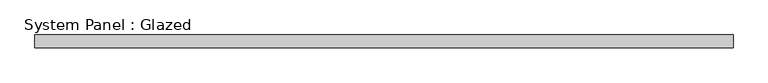
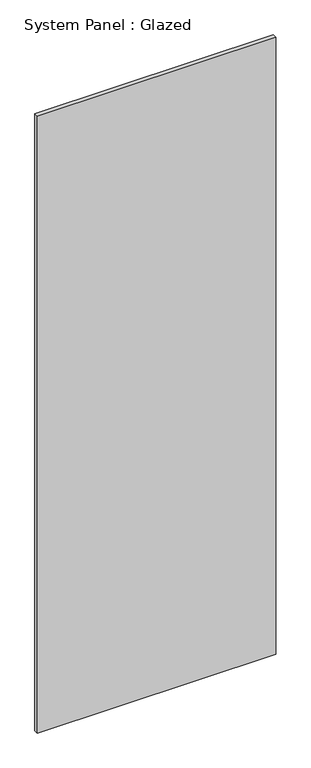
"""IFC4 building model written with IfcOpenShell, lengths in millimetres: plate geometry, System Panel : Glazed."""

from ifc_helpers import new_model, si_unit, origin, origin_with_axes, place, context, project, spatial, polyline, outline, extrude, source, transform, mapped, element, save


def system_panel_glazed_b761a9a7(model_context):
    return source(origin(), model_context, "Body", "SweptSolid", [
        extrude(outline(polyline([(698.5, 19.05), (-698.5, 19.05), (-698.5, 44.45), (698.5, 44.45), (698.5, 19.05)])), origin_with_axes(), (0.0, 0.0, 1.0), 3824.2205189),
    ])


if __name__ == "__main__":
    model = new_model("IFC4")
    model_context = context("Model", 3, world=origin())
    ifc_project = project(units=[si_unit("LENGTHUNIT", "METRE", prefix="MILLI")], contexts=[model_context])
    site = spatial("IfcSite", under=ifc_project)
    building = spatial("IfcBuilding", under=site)
    placement = place(None, origin())
    system_panel_glazed_shape = system_panel_glazed_b761a9a7(model_context)
    element("IfcPlate", 1, ObjectType="System Panel : Glazed", at=placement, inside=building, context=model_context, shape_type="MappedRepresentation", body=[
        mapped(system_panel_glazed_shape, transform((0.0, 0.0, 0.0), x_axis=(1.0, 0.0, 0.0), y_axis=(0.0, 1.0, 0.0), z_axis=(0.0, 0.0, 1.0))),
    ])
    save(model, "model.ifc")

# Revit data of these elements
# Type "System Panel : Glazed"
#   Construction Type Id = "GSP4R"
#   Analytic Construction = "1/8 in Pilkington single glazing"
#   Visual Light Transmittance = 0.9
#   Solar Heat Gain Coefficient = 0.86
#   Heat Transfer Coefficient (U) = 1.18115 BTU/(h·ft²·°F)
#   Define Thermal Properties by = 1
# Element 1 (IfcPlate, "System Panel : Glazed")
#   Materials on its faces: "Glass"
# Materials
#   "Glass": class "Glass", colour RGB 0 128 192, transparency 0.75, Description = "Soda Lime Glass", Cost = 0
